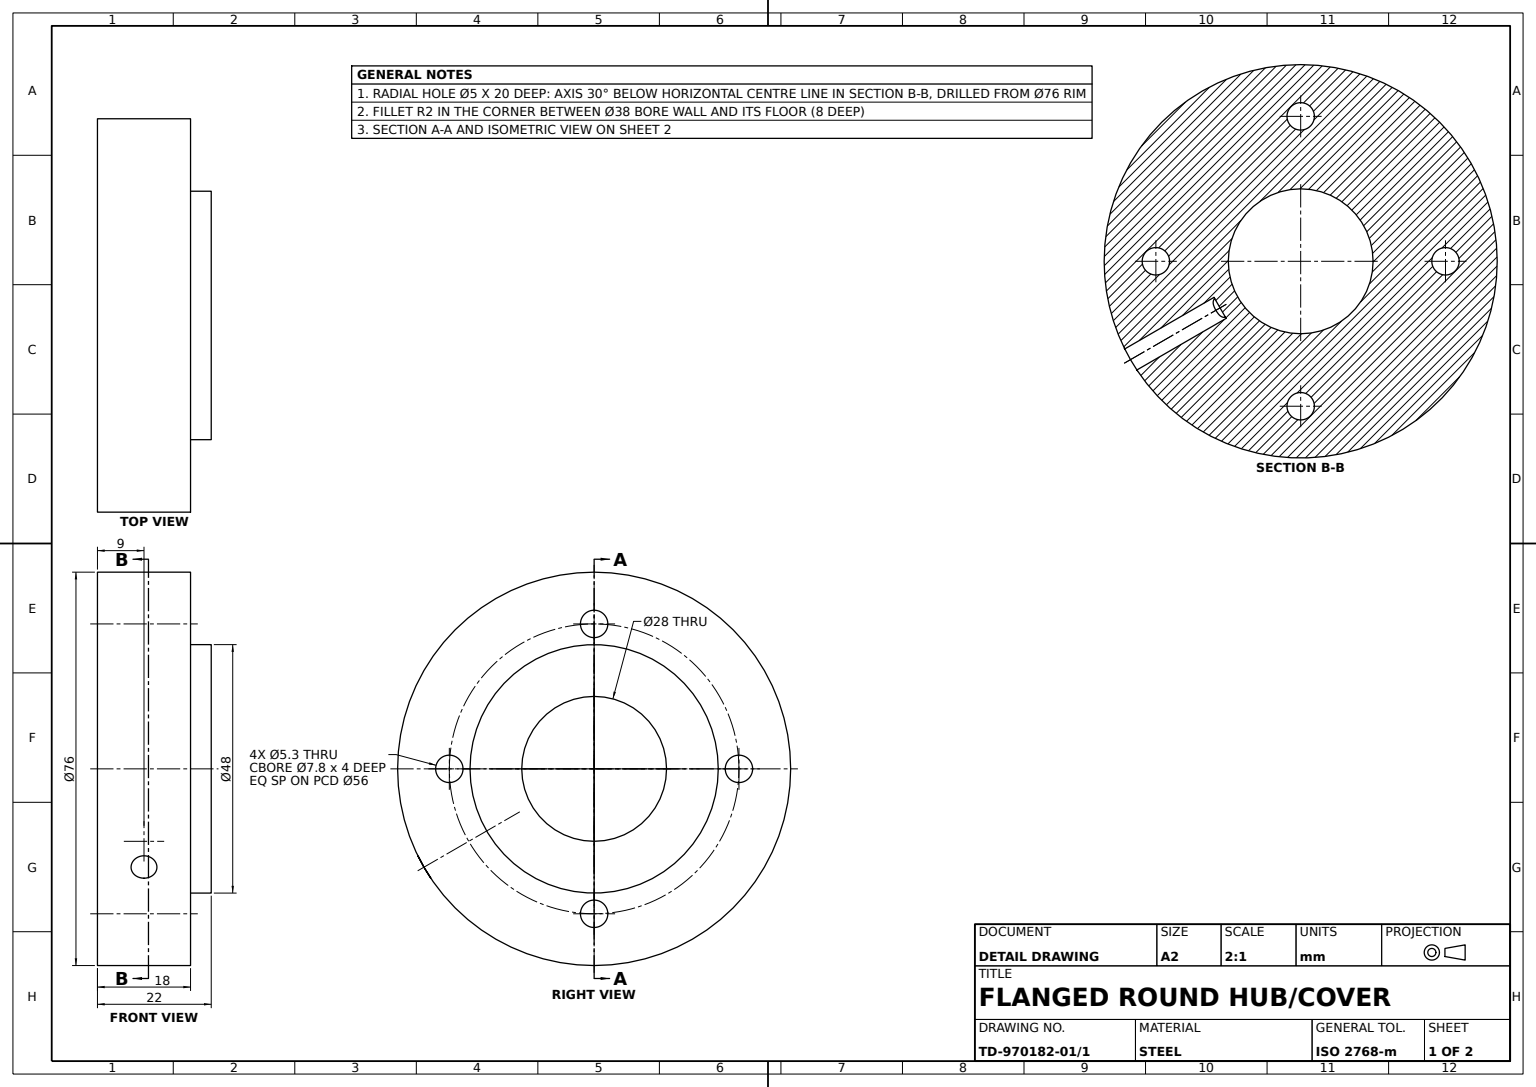
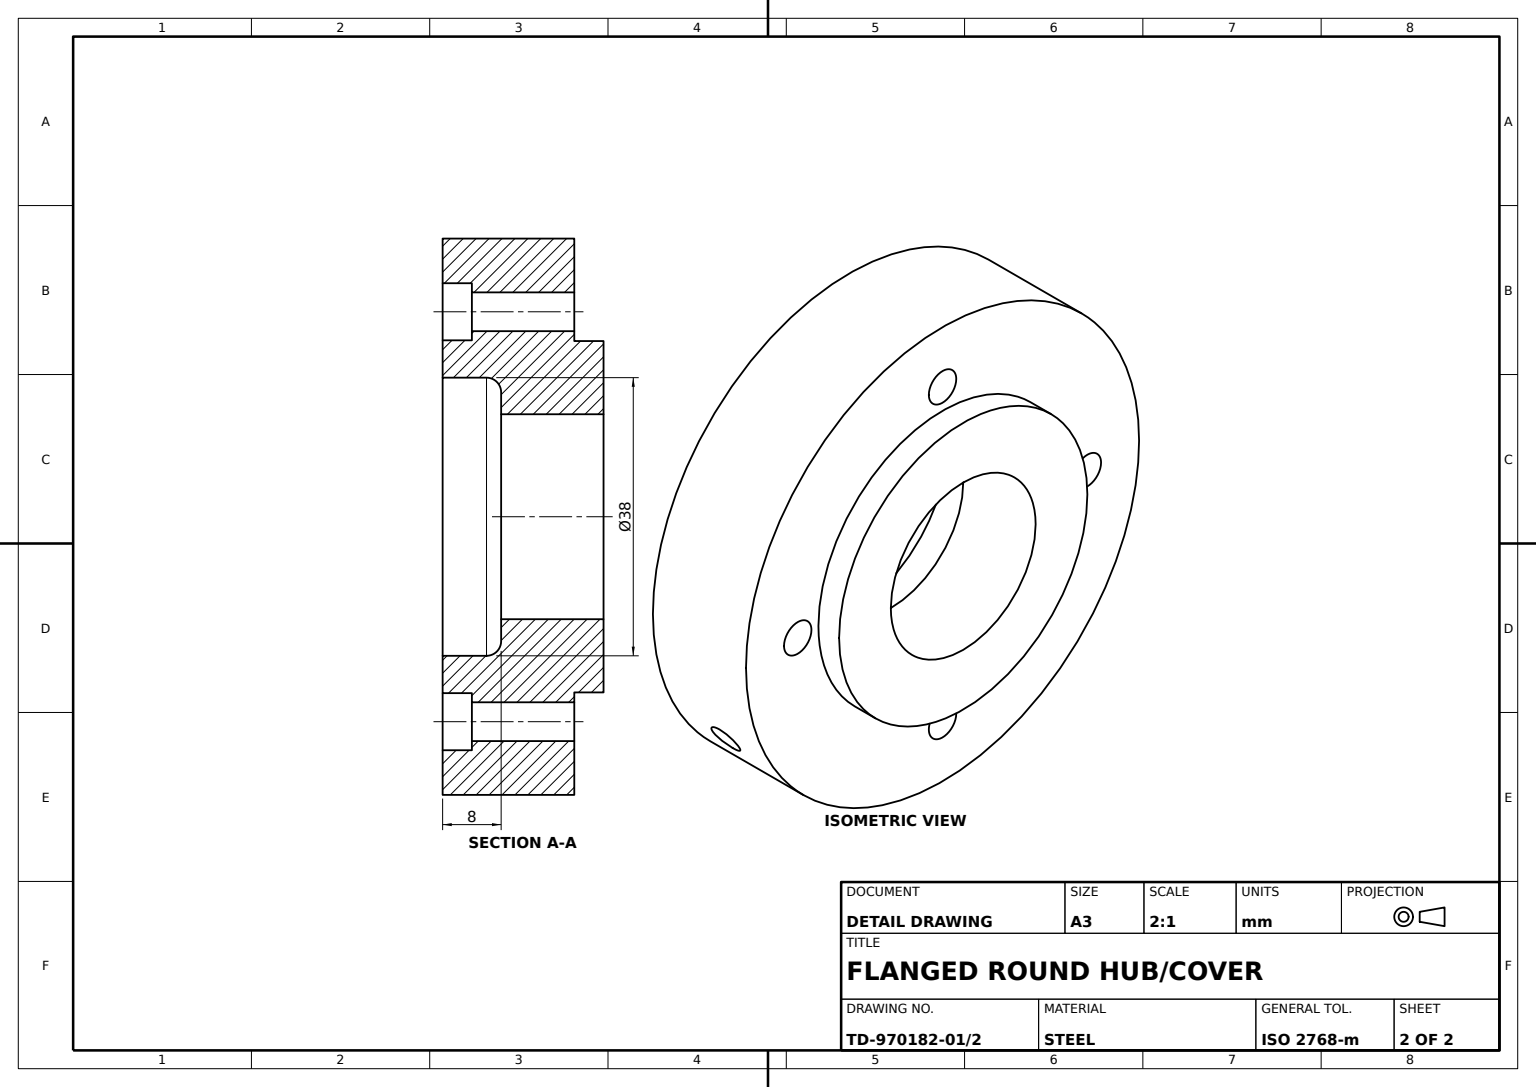
from build123d import *

# Parameters (mm, degrees)
BASE_DISC_SKETCH_R                          = 38
BASE_DISC_76X18_DEPTH                       = 9
SPIGOT_SKETCH_R                             = 24
SPIGOT_48X8_DEPTH                           = 4
COUNTERBORED_MOUNTING_HOLES_5_3_D           = 5.3
COUNTERBORED_MOUNTING_HOLES_5_3_CBORE_D     = 7.8
COUNTERBORED_MOUNTING_HOLES_5_3_CBORE_DEPTH = 4
COUNTERBORE_BORE_SKETCH_R                   = 19
COUNTERBORE_BORE_38X16_DEPTH                = 8
THROUGH_BORE_28_REACH                       = 57.534
THROUGH_BORE_SKETCH_R                       = 14
BORE_EDGE_FILLET_R2_R                       = 2
RADIAL_HOLE_5X20_D                          = 5
RADIAL_HOLE_5X20_DEPTH                      = 20


with BuildPart() as part:
    # Base Disc Sketch → Base Disc Ø76x18 (new, symmetric)
    with BuildSketch(Plane(origin=(0, 0, 0), x_dir=(1, 0, 0), z_dir=(0, 1, 0))):
        with Locations(Location((0, 0, 0), (0, 0, 270))):
            Circle(BASE_DISC_SKETCH_R)
    extrude(amount=BASE_DISC_76X18_DEPTH, both=True)

    # Spigot Sketch → Spigot Ø48x8 (add, symmetric)
    with BuildSketch(Plane(origin=(0, 9, 0), x_dir=(1, 0, 0), z_dir=(0, 1, 0))):
        with Locations(Location((0, 0, 0), (0, 0, 270))):
            Circle(SPIGOT_SKETCH_R)
    extrude(amount=SPIGOT_48X8_DEPTH, both=True)

    # Counterbored Mounting Holes Ø5.3 (through all)
    with Locations(Plane(origin=(0, -9, 28), x_dir=(0, 0, -1), z_dir=(0, -1, 0))):
        with Locations((0, 0), (28, 28), (56, 0), (28, -28)):
            CounterBoreHole(COUNTERBORED_MOUNTING_HOLES_5_3_D / 2, COUNTERBORED_MOUNTING_HOLES_5_3_CBORE_D / 2, COUNTERBORED_MOUNTING_HOLES_5_3_CBORE_DEPTH)

    # Counterbore Bore Sketch → Counterbore Bore Ø38x16 (cut, symmetric)
    with BuildSketch(Plane.XZ.offset(9)):
        with Locations(Location((0, 0, 0), (0, 0, 270))):
            Circle(COUNTERBORE_BORE_SKETCH_R)
    extrude(amount=COUNTERBORE_BORE_38X16_DEPTH, both=True, mode=Mode.SUBTRACT)

    # Through Bore Sketch → Through Bore Ø28 (cut, up to next)
    with BuildSketch(Plane.XZ.offset(1), mode=Mode.PRIVATE) as through_bore_28_sk1:
        with Locations(Location((0, 0, 0), (0, 0, 270))):
            Circle(THROUGH_BORE_SKETCH_R)
    through_bore_28_tool1 = extrude(through_bore_28_sk1.sketch, amount=-THROUGH_BORE_28_REACH, mode=Mode.PRIVATE) & part.part
    add(through_bore_28_tool1.solids().sort_by_distance((0, -1, 0))[0], mode=Mode.SUBTRACT)

    # Bore Edge Fillet R2
    bore_edge_fillet_r2_edges = [part.edges().sort_by_distance(p)[0] for p in [
        (0, -1, 19),
    ]]
    fillet(bore_edge_fillet_r2_edges, radius=BORE_EDGE_FILLET_R2_R)

    # Radial Hole Ø5x20
    with Locations(Plane(origin=(19, 0, 32.908965344), x_dir=(0.8660254037844379, 0, -0.5000000000000013), z_dir=(0.5000000000000013, 0, 0.8660254037844379))):
        with Locations((0, 0)):
            Hole(RADIAL_HOLE_5X20_D / 2, depth=RADIAL_HOLE_5X20_DEPTH)


solid = part.part
